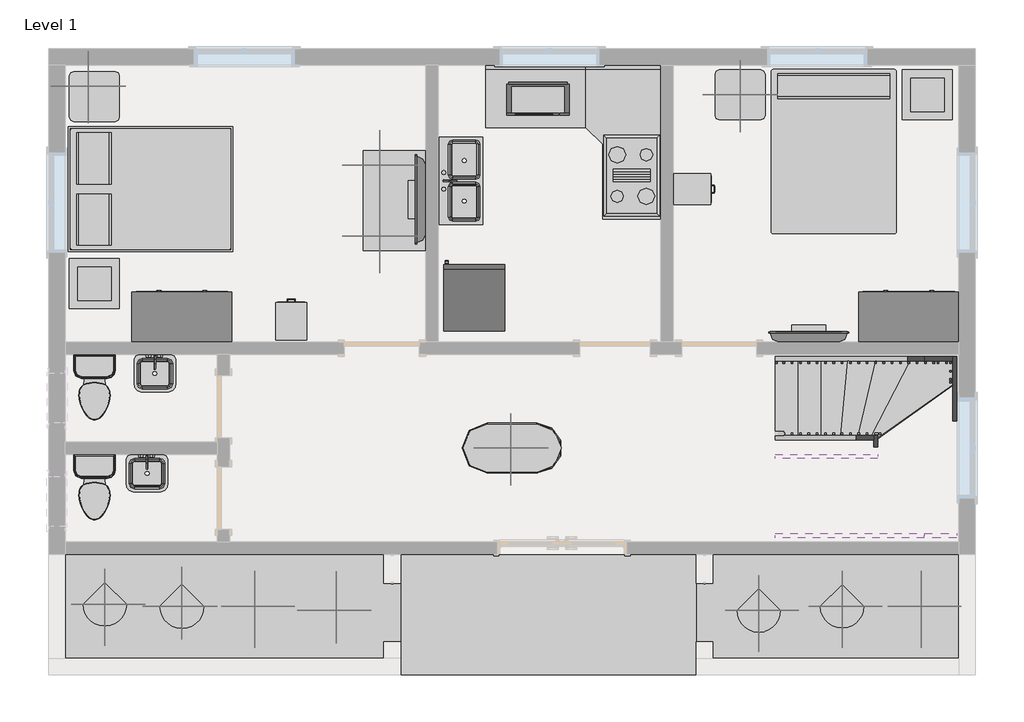
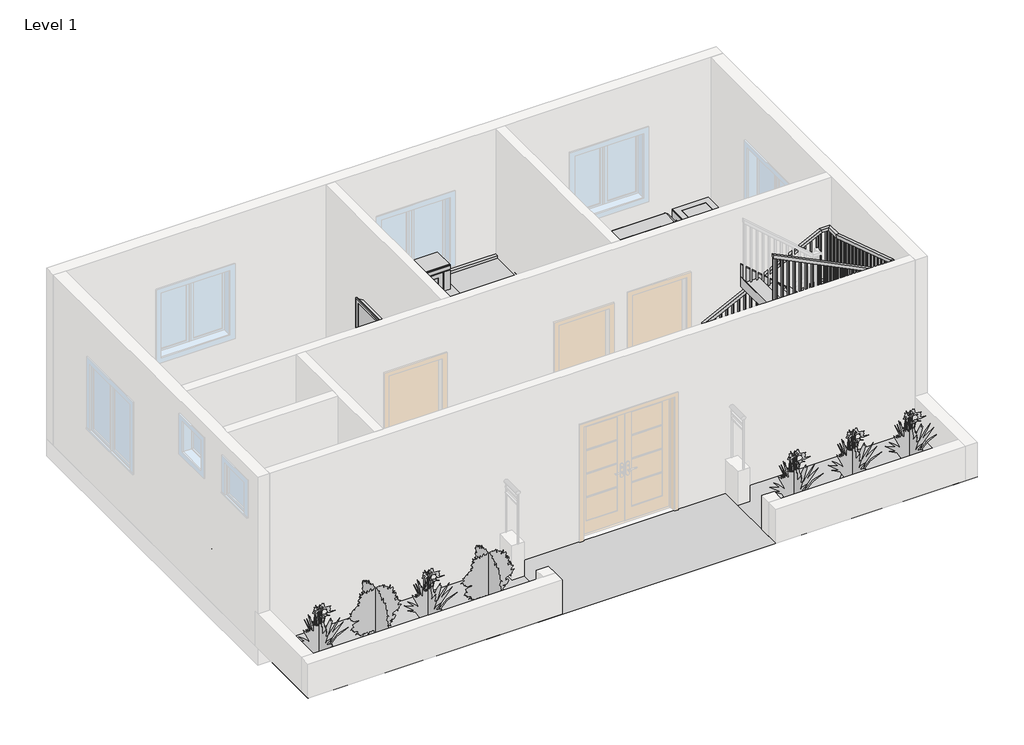
# One storey, part 2 of 2: 15 furniture elements, 12 geographic elements, 8 members, 7 flow terminals, 6 proxies, 1 railing, 1 stair flight.
# Revit data of these elements (continued)
# Element 5 (IfcBuildingElementProxy, "Microwave : 30\" x 16\" x 18\"") (continued)
#   Phase Created = New Construction
#   Materials on its faces: "Laminate - Ivory, Glossy", "Glass"
# Element 6 (IfcBuildingElementProxy, "Refrigerator : 30\" x 32\" RH")
#   Phase Created = New Construction
#   Materials on its faces: "Copper", "Steel, Chrome Plated"
# Element 7 (IfcFlowTerminal, "Floor Drain - Round : 5\" Strainer - 2\" Drain")
#   Mark = "7"
#   Phase Created = New Construction
# Element 8 (IfcFlowTerminal, "Floor Drain - Round : 5\" Strainer - 2\" Drain")
#   Mark = "8"
#   Phase Created = New Construction
# Element 9 (IfcFlowTerminal, "Sink Kitchen-Double : 42\" x 21\"")
#   Mark = "2"
#   Phase Created = New Construction
#   Materials on its faces: "Steel, Polished"
# Element 10 (IfcFlowTerminal, "Sink Vanity-Square : 20\" x 18\"")
#   Mark = "4"
#   Phase Created = New Construction
#   Materials on its faces: "Porcelain, Linen", "Steel, Polished"
# Element 11 (IfcFlowTerminal, "Sink Vanity-Square : 20\" x 18\"")
#   Mark = "6"
#   Phase Created = New Construction
#   Materials on its faces: "Porcelain, Linen", "Steel, Polished"
# Element 12 (IfcFlowTerminal, "Toilet-Domestic-3D : Toilet-Domestic-3D")
#   Mark = "3"
#   Phase Created = New Construction
#   Materials on its faces: "Porcelain, Linen", "Laminate, Linen, Matte"
# Element 13 (IfcFlowTerminal, "Toilet-Domestic-3D : Toilet-Domestic-3D")
#   Mark = "5"
#   Phase Created = New Construction
#   Materials on its faces: "Porcelain, Linen", "Laminate, Linen, Matte"
# Element 14 (IfcFurniture, "Bed-Box : Queen 60\" x 79\"")
#   Phase Created = New Construction
#   Materials on its faces: "Birch", "Sash"
# Element 15 (IfcFurniture, "Bed-Standard.0001 : Queen 60\" x 79\"")
#   Phase Created = New Construction
#   Materials on its faces: "Linen, White", "Steel, Chrome Plated"
# Elements 16, 17 (IfcFurniture, "Cabinet-File 2 Drawer : 15\" x 18\"")
#   Phase Created = New Construction
#   Materials on its faces: "Steel, Chrome Plated", "Steel, Paint Finish, Ivory, Glossy"
# Elements 18, 19 (IfcFurniture, "Dresser : 48\" x 72\" x 24\"")
#   Phase Created = New Construction
#   Materials on its faces: "Laminate, Ivory, Matte", "Cherry", "Wood - Teak"
# Element 20 (IfcFurniture, "TV - Flat Screen : 37\"")
#   Stand = yes
#   Phase Created = New Construction
#   Materials on its faces: "TV - Black", "TV - Glass", "TV - Screen"
# Element 21 (IfcFurniture, "TV - Flat Screen : 42\"")
#   Stand = yes
#   Phase Created = New Construction
#   Materials on its faces: "TV - Black", "TV - Glass", "TV - Screen"
# Elements 22, 23 (IfcFurniture, "Table-Coffee : 24\" x 24\" x 24\"")
#   Phase Created = New Construction
#   Materials on its faces: "Glass - Clear, Grey"
# Element 24 (IfcFurniture, "Table-Dining Oval : 36\" x 48\"")
#   Phase Created = New Construction
#   Materials on its faces: "Steel, Chrome Plated", "Glass - Clear, Grey"
# Elements 25, 26 (IfcFurniture, "Table-End : 24\" x 24\"")
#   Phase Created = New Construction
#   Materials on its faces: "Laminate, Ivory, Matte", "Birch"
# Element 27 (IfcFurniture, "Table-Rectangular : 72\" x 30\"")
#   Phase Created = New Construction
#   Materials on its faces: "Birch"
# Element 28 (IfcFurniture, "Work Station Cubicle : 96\" x 96\"")
#   Phase Created = New Construction
#   Materials on its faces: "Textile - Light Gray", "Laminate, Ivory, Matte"
# Elements 29, 30, 31, 32, 33 (IfcGeographicElement, "RPC Plant - Tropical")
#   Phase Created = New Construction
# Elements 34, 35, 36, 37, 38 (IfcGeographicElement, "RPC Plant - Tropical : Agave - 1.5'")
#   Phase Created = New Construction
# Elements 39, 40 (IfcGeographicElement, "RPC Plant - Tropical : Jungle Flame - 3'")
#   Phase Created = New Construction
# Elements 41, 42, 43, 44, 45, 46, 47, 48 (IfcMember, "Stringer - 2\" Width")
#   Phase Created = New Construction
# Element 49 (IfcRailing, "Handrail - Rectangular")
#   Phase Created = New Construction
# Element 50 (IfcStairFlight, "2\" Tread 1\" Nosing 1/4\" Riser")
#   Phase Created = New Construction
# Materials
#   "Steel, Chrome Plated": class "Metal", colour RGB 17 17 17, transparency 0, Description = "Chromiuim plated steel", Cost = 0
#   "Steel, Polished": class "Metal", colour RGB 57 57 57, transparency 0, Description = "Polished steel", Cost = 0
#   "Laminate - Ivory, Glossy": colour RGB 247 247 239, transparency 0
#   "Copper": class "Metal", colour RGB 0 0 0, transparency 0, Description = "Copper, matte finish", Cost = 0
#   "Porcelain, Linen": class "Ceramic", colour RGB 249 239 230, transparency 0, Description = "Porcelain, linen", Cost = 0
#   "Laminate, Linen, Matte": class "Plastic", colour RGB 249 239 230, transparency 0, Description = "Plastic Laminate - Linen, Matte", Cost = 0
#   "Birch": class "Wood", colour RGB 224 178 126, transparency 0, Description = "Betula Alleghaniensis", Cost = 0
#   "Sash": class "Wood", colour RGB 224 178 126, transparency 0
#   "Linen, White": class "Textile", colour RGB 247 247 239, transparency 0, Description = "Linen, white", Cost = 0
#   "Steel, Paint Finish, Ivory, Glossy": class "Metal", colour RGB 247 247 239, transparency 0, Description = "Steel, paint finish, ivory, glossy", Cost = 0
#   "Wood - Teak": class "Wood", colour RGB 145 112 90, transparency 0
#   "Laminate, Ivory, Matte": class "Plastic", colour RGB 247 247 239, transparency 0, Description = "Plastic Laminate - Ivory, Matte", Cost = 0
#   "Cherry": class "Wood", colour RGB 226 177 128, transparency 0, Description = "Prunus Serotina", Cost = 0
#   "Glass - Clear, Grey": class "Glass", colour RGB 252 255 255, transparency 0.64
#   "Textile - Light Gray": class "Fabric", colour RGB 204 204 204, transparency 0
#   "Plant": class "Generic", colour RGB 0 0 0, transparency 0, Description = "physical material", Cost = 0
#   "Concrete": class "Concrete", colour RGB 0 0 0, transparency 0, Description = "Portland Cement Concrete", Cost = 0
#   "Glass": class "Glass", colour RGB 0 128 192, transparency 0.75, Description = "Soda Lime Glass", Cost = 0
#   "TV - Black": colour RGB 49 49 49, transparency 0
#   "TV - Glass": colour RGB 157 157 157, transparency 0.9
#   "TV - Screen": colour RGB 0 0 0, transparency 0
